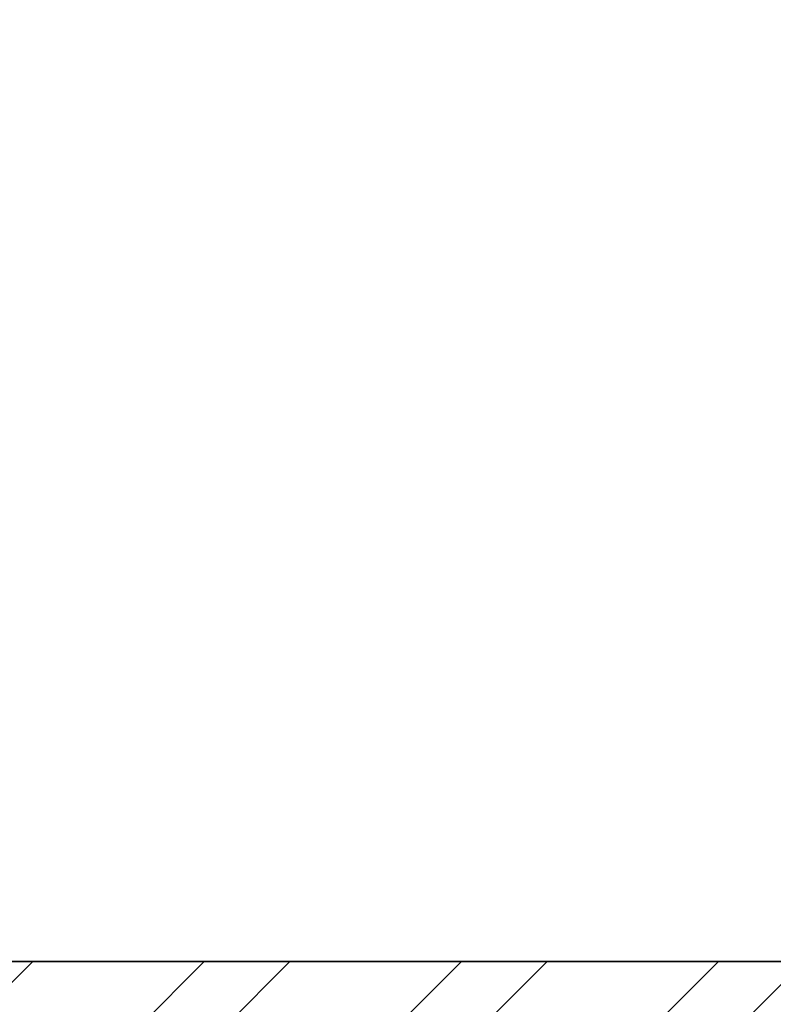
# Model space of a CAD drawing. Units: inches. Extents: x 1962 to 2771, y 1245 to 2660.
# Tile 71 of 114: x 2551 to 2590, y 1979 to 2031. Entities that reach past the tile are written whole.
import ezdxf

# ---------------------------------------------------------------- set-up
doc = ezdxf.new("R2010")
doc.units = ezdxf.units.IN
doc.layers.add('A-WALL', color=7, linetype='Continuous', lineweight=35)
doc.layers.add('A-WALL-PATT', color=252, linetype='Continuous', lineweight=13)

msp = doc.modelspace()

# ---------------------------------------------------------------- hatches: boundary and pattern name
at = {"layer": 'A-WALL-PATT'}
h = msp.add_hatch(dxfattribs=at)
h.set_pattern_fill('ANSI32', color=256)
h.paths.add_polyline_path([(2090.8074, 2467.3437), (2141.6481, 2467.3437), (2141.6481, 2469.5937), (2141.6481, 2471.8437), (2086.3074, 2471.8437), (2086.3074, 2422.5333), (2090.8074, 2422.5333)])
h.paths.add_polyline_path([(2282.7664, 2471.8437), (2204.8982, 2471.8437), (2204.8982, 2467.3437), (2234.8074, 2467.3437), (2234.8074, 2311.3437), (2228.7492, 2311.3437), (2228.7492, 2306.8437), (2234.8074, 2306.8437), (2331.9227, 2306.8437), (2331.9227, 2309.0937), (2331.9227, 2311.3437), (2239.3074, 2311.3437), (2239.3074, 2467.3437), (2282.7664, 2467.3437), (2282.7664, 2469.5937)])
h.paths.add_polyline_path([(2471.4531, 2519.8437), (2552.011, 2519.8437), (2564.3996, 2519.8437), (2564.3996, 2511.1389), (2568.8996, 2511.1389), (2568.8996, 2524.3437), (2466.9531, 2524.3437), (2466.9531, 2471.8437), (2450.0749, 2471.8437), (2446.4672, 2471.8437), (2446.4672, 2467.3437), (2450.0749, 2467.3437), (2475.9988, 2467.3437), (2475.9988, 2469.5937), (2475.9988, 2471.8437), (2471.4531, 2471.8437)])
h.paths.add_polyline_path([(2575.2231, 2469.5937), (2575.2231, 2471.8437), (2568.8996, 2471.8437), (2568.8996, 2487.1389), (2564.3996, 2487.1389), (2564.3996, 2471.8437), (2556.511, 2471.8437), (2499.2904, 2471.8437), (2499.2904, 2467.3437), (2507.8074, 2467.3437), (2507.8074, 2311.3437), (2414.863, 2311.3437), (2414.863, 2306.8437), (2512.3074, 2306.8437), (2517.0114, 2306.8437), (2517.0114, 2309.0937), (2517.0114, 2311.3437), (2512.3074, 2311.3437), (2512.3074, 2467.3437), (2575.2231, 2467.3437)])
h.paths.add_polyline_path([(2660.8074, 2471.8437), (2600.9602, 2471.8437), (2600.9602, 2467.3437), (2656.3074, 2467.3437), (2656.3074, 2432.5704), (2660.8074, 2432.5704)])
h.paths.add_polyline_path([(2660.8074, 2372.5704), (2656.3074, 2372.5704), (2656.3074, 2311.3437), (2600.276, 2311.3437), (2600.276, 2309.0937), (2600.276, 2306.8437), (2656.3074, 2306.8437), (2656.3074, 2296.2593), (2660.8074, 2296.2593)])
h.paths.add_polyline_path([(2572.3074, 2306.8437), (2577.1385, 2306.8437), (2577.1385, 2311.3437), (2551.082, 2311.3437), (2551.082, 2306.8437), (2567.8074, 2306.8437), (2567.8074, 2258.8437), (2540.0574, 2258.8437), (2540.0574, 2256.5937), (2540.0574, 2254.3437), (2567.8074, 2254.3437), (2656.3074, 2254.3437), (2656.3074, 2236.9085), (2660.8074, 2236.9085), (2660.8074, 2272.2593), (2656.3074, 2272.2593), (2656.3074, 2258.8437), (2572.3074, 2258.8437)])
h.paths.add_polyline_path([(2512.3074, 2254.3437), (2518.8716, 2254.3437), (2518.8716, 2256.5937), (2518.8716, 2258.8437), (2507.8074, 2258.8437), (2507.8074, 2177.8437), (2567.8074, 2177.8437), (2567.8074, 2172.9628), (2572.3074, 2172.9628), (2572.3074, 2177.8437), (2656.3074, 2177.8437), (2656.3074, 2166.4846), (2660.8074, 2166.4846), (2660.8074, 2200.9085), (2656.3074, 2200.9085), (2656.3074, 2182.3437), (2512.3074, 2182.3437)])
h.paths.add_polyline_path([(2656.3074, 2129.8437), (2572.3074, 2129.8437), (2572.3074, 2150.3044), (2570.0574, 2150.3044), (2567.8074, 2150.3044), (2567.8074, 2129.8437), (2507.8074, 2129.8437), (2507.8074, 2116.3027), (2510.0574, 2116.3027), (2512.3074, 2116.3027), (2512.3074, 2125.3437), (2567.8074, 2125.3437), (2572.3074, 2125.3437), (2656.3074, 2125.3437)])
h.paths.add_polyline_path([(2090.8074, 2362.5333), (2086.3074, 2362.5333), (2086.3074, 2298.6242), (2090.8074, 2298.6242), (2090.8074, 2306.8437), (2174.8074, 2306.8437), (2174.8074, 2286.4178), (2179.3074, 2286.4178), (2179.3074, 2306.8437), (2192.8641, 2306.8437), (2192.8641, 2309.0937), (2192.8641, 2311.3437), (2090.8074, 2311.3437)])
h.paths.add_polyline_path([(2209.156, 2258.8437), (2179.3074, 2258.8437), (2179.3074, 2263.2236), (2177.0574, 2263.2236), (2174.8074, 2263.2236), (2174.8074, 2258.8437), (2090.8074, 2258.8437), (2090.8074, 2274.6242), (2086.3074, 2274.6242), (2086.3074, 2238.2967), (2088.5574, 2238.2967), (2090.8074, 2238.2967), (2090.8074, 2254.3437), (2209.156, 2254.3437)])
h.paths.add_polyline_path([(2090.8074, 2177.8437), (2234.8074, 2177.8437), (2234.8074, 2173.1428), (2239.3074, 2173.1428), (2239.3074, 2258.8437), (2230.8442, 2258.8437), (2230.8442, 2256.5937), (2230.8442, 2254.3437), (2234.8074, 2254.3437), (2234.8074, 2182.3437), (2090.8074, 2182.3437), (2090.8074, 2202.2967), (2086.3074, 2202.2967), (2086.3074, 2140.0389), (2090.8074, 2140.0389)])
h.paths.add_polyline_path([(2090.8074, 2080.0389), (2086.3074, 2080.0389), (2086.3074, 2033.8437), (2090.8074, 2033.8437)], flags=17)
h.paths.add_polyline_path([(2244.9405, 2033.8437), (2239.3074, 2033.8437), (2239.3074, 2142.0665), (2237.2592, 2142.0665), (2234.8074, 2142.0665), (2234.8074, 2033.8437), (2090.8074, 2033.8437), (2076.5204, 2033.8437), (2072.0204, 2033.8437), (2072.0204, 2000.4493), (2076.5204, 2000.4493), (2076.5204, 2029.3437), (2090.8074, 2029.3437), (2244.9405, 2029.3437), (2244.9405, 2031.5937)])
h.paths.add_polyline_path([(2234.8074, 1933.3437), (2076.5204, 1933.3437), (2076.5204, 1952.4493), (2074.2704, 1952.4493), (2072.0204, 1952.4493), (2072.0204, 1933.3437), (2072.0204, 1928.8437), (2234.8074, 1928.8437)])
h.paths.add_polyline_path([(2090.8074, 1928.8437), (2086.3074, 1928.8437), (2086.3074, 1906.5013), (2090.8074, 1906.5013)])
h.paths.add_polyline_path([(2090.8074, 1846.5013), (2086.3074, 1846.5013), (2086.3074, 1769.9917), (2088.5574, 1769.9917), (2090.8074, 1769.9917), (2090.8074, 1780.3437), (2234.8074, 1780.3437), (2234.8074, 1708.3437), (2230.3764, 1708.3437), (2230.3764, 1703.8437), (2239.3074, 1703.8437), (2239.3074, 1792.6669), (2237.0574, 1792.6669), (2234.8074, 1792.6669), (2234.8074, 1784.8437), (2090.8074, 1784.8437)])
h.paths.add_polyline_path([(2239.3074, 1928.8437), (2244.9405, 1928.8437), (2244.9405, 1931.0937), (2244.9405, 1933.3437), (2234.8074, 1933.3437), (2234.8074, 1928.8437), (2234.8074, 1825.5949), (2239.3074, 1825.5949)])
h.paths.add_polyline_path([(2148.0425, 1649.0937), (2148.0425, 1651.3437), (2090.8074, 1651.3437), (2090.8074, 1646.8437), (2148.0425, 1646.8437)], flags=0)
h.paths.add_polyline_path([(2207.5601, 1708.3437), (2090.8074, 1708.3437), (2090.8074, 1703.8437), (2174.8074, 1703.8437), (2174.8074, 1651.3437), (2170.4457, 1651.3437), (2170.4457, 1646.8437), (2195.9924, 1646.8437), (2195.9924, 1649.0937), (2195.9924, 1651.3437), (2179.3074, 1651.3437), (2179.3074, 1703.8437), (2207.5601, 1703.8437), (2207.5601, 1706.0937)])
h.paths.add_polyline_path([(2090.8074, 1733.9917), (2086.3074, 1733.9917), (2086.3074, 1696.1032), (2088.5574, 1696.1032), (2090.8074, 1696.1032)])
h.paths.add_polyline_path([(2090.8074, 1672.1032), (2086.3074, 1672.1032), (2086.3074, 1600.3335), (2090.8074, 1600.3335)])
h.paths.add_polyline_path([(2090.8074, 1540.3335), (2086.3074, 1540.3335), (2086.3074, 1486.3437), (2139.6766, 1486.3437), (2139.6766, 1490.8437), (2090.8074, 1490.8437)])
h.paths.add_polyline_path([(2302.3876, 1490.8437), (2239.3074, 1490.8437), (2239.3074, 1646.8437), (2335.9994, 1646.8437), (2335.9994, 1651.3437), (2229.884, 1651.3437), (2229.884, 1646.8437), (2234.8074, 1646.8437), (2234.8074, 1490.8437), (2202.7103, 1490.8437), (2202.7103, 1488.5937), (2202.7103, 1486.3437), (2275.0699, 1486.3437), (2275.0699, 1475.772), (2279.5699, 1475.772), (2279.5699, 1486.3437), (2302.3876, 1486.3437)])
h.paths.add_polyline_path([(2279.5699, 1451.772), (2275.0699, 1451.772), (2275.0699, 1438.3437), (2174.8074, 1438.3437), (2174.8074, 1486.3437), (2179.7922, 1486.3437), (2179.7922, 1490.8437), (2163.3585, 1490.8437), (2163.3585, 1488.5937), (2163.3585, 1486.3437), (2170.3074, 1486.3437), (2170.3074, 1433.8437), (2279.5699, 1433.8437)])
h.paths.add_polyline_path([(2427.2363, 1490.8437), (2375.8074, 1490.8437), (2375.8074, 1646.8437), (2381.6401, 1646.8437), (2381.6401, 1651.3437), (2365.887, 1651.3437), (2365.887, 1649.0937), (2365.887, 1646.8437), (2371.3074, 1646.8437), (2371.3074, 1490.8437), (2327.5627, 1490.8437), (2327.5627, 1488.5937), (2327.5627, 1486.3437), (2371.3074, 1486.3437), (2371.3074, 1433.8437), (2375.8074, 1433.8437), (2375.8074, 1486.3437), (2427.2363, 1486.3437)])
h.paths.add_polyline_path([(2512.3074, 1646.8437), (2519.4351, 1646.8437), (2519.4351, 1649.0937), (2519.4351, 1651.3437), (2507.8074, 1651.3437), (2416.0063, 1651.3437), (2416.0063, 1649.0937), (2416.0063, 1646.8437), (2507.8074, 1646.8437), (2507.8074, 1490.8437), (2497.0532, 1490.8437), (2497.0532, 1488.5937), (2497.0532, 1486.3437), (2574.9344, 1486.3437), (2574.9344, 1476.0181), (2579.4344, 1476.0181), (2579.4344, 1486.3437), (2584.4872, 1486.3437), (2584.3074, 1490.8437), (2512.3074, 1490.8437)])
h.paths.add_polyline_path([(2470.5091, 1486.3437), (2473.9767, 1486.3437), (2473.9767, 1490.8437), (2449.6605, 1490.8437), (2449.6605, 1488.5937), (2449.6605, 1486.3437), (2466.0091, 1486.3437), (2466.0091, 1433.8437), (2470.5091, 1433.8437), (2579.4344, 1433.8437), (2579.4344, 1452.0181), (2574.9344, 1452.0181), (2574.9344, 1438.3437), (2554.5091, 1438.3437), (2470.5091, 1438.3437)])
h.paths.add_polyline_path([(2656.3074, 1490.8437), (2611.86, 1490.8437), (2611.86, 1486.3437), (2656.3074, 1486.3437)])
h.paths.add_polyline_path([(2660.8074, 1532.7007), (2658.5574, 1532.7007), (2656.3074, 1532.7007), (2656.3074, 1486.3437), (2660.8074, 1486.3437)])
h.paths.add_polyline_path([(2660.8074, 1664.9663), (2656.3074, 1664.9663), (2656.3074, 1651.3437), (2602.2313, 1651.3437), (2602.2313, 1646.8437), (2656.3074, 1646.8437), (2656.3074, 1592.7007), (2660.8074, 1592.7007)])
h.paths.add_polyline_path([(2660.8074, 1724.5221), (2656.3074, 1724.5221), (2656.3074, 1703.8437), (2542.4725, 1703.8437), (2542.4725, 1699.3437), (2567.8074, 1699.3437), (2567.8074, 1651.3437), (2552.7766, 1651.3437), (2552.7766, 1649.0937), (2552.7766, 1646.8437), (2577.2878, 1646.8437), (2577.2878, 1649.0937), (2577.2878, 1651.3437), (2572.3074, 1651.3437), (2572.3074, 1699.3437), (2656.3074, 1699.3437), (2656.3074, 1688.9663), (2660.8074, 1688.9663)])
h.paths.add_polyline_path([(2660.8074, 1880.6524), (2656.3074, 1880.6524), (2656.3074, 1832.8437), (2512.3074, 1832.8437), (2512.3074, 1837.8959), (2507.8074, 1837.8959), (2507.8074, 1828.3437), (2567.8074, 1828.3437), (2567.8074, 1804.3437), (2572.3074, 1804.3437), (2572.3074, 1828.3437), (2656.3074, 1828.3437), (2656.3074, 1818.6778), (2660.8074, 1818.6778)])
h.paths.add_polyline_path([(2660.8074, 1794.6778), (2656.3074, 1794.6778), (2656.3074, 1780.3437), (2572.3074, 1780.3437), (2572.3074, 1783.0303), (2570.0574, 1783.0303), (2567.8074, 1783.0303), (2567.8074, 1780.3437), (2507.8074, 1780.3437), (2507.8074, 1699.3437), (2517.8858, 1699.3437), (2517.8858, 1701.5937), (2517.8858, 1703.8437), (2512.3074, 1703.8437), (2512.3074, 1775.8437), (2656.3074, 1775.8437), (2656.3074, 1760.5221), (2660.8074, 1760.5221)])
h.paths.add_polyline_path([(2660.8074, 1981.3437), (2660.8074, 2020.2808), (2658.5574, 2020.2808), (2656.3074, 2020.2808), (2656.3074, 1981.3437), (2512.3074, 1981.3437), (2512.3074, 2086.6996), (2507.8074, 2086.6996), (2507.8074, 1981.3437), (2375.8074, 1981.3437), (2375.8074, 1986.8505), (2373.5574, 1986.8505), (2371.3074, 1986.8505), (2371.3074, 1973.2607), (2375.8074, 1973.2607), (2375.8074, 1976.8437), (2507.8074, 1976.8437), (2507.8074, 1865.4281), (2510.0574, 1865.4281), (2512.3074, 1865.4281), (2512.3074, 1976.8437), (2660.8074, 1976.8437)])
h.paths.add_polyline_path([(2375.8074, 1940.297), (2373.5574, 1940.297), (2371.3074, 1940.297), (2371.3074, 1933.3437), (2278.4434, 1933.3437), (2278.4434, 1928.8437), (2371.3074, 1928.8437), (2371.3074, 1651.3437), (2375.8074, 1651.3437)])
h.paths.add_polyline_path([(2660.8074, 1976.8437), (2656.3074, 1976.8437), (2656.3074, 1940.6524), (2660.8074, 1940.6524)], flags=17)
h.paths.add_polyline_path([(2660.8074, 2142.4846), (2656.3074, 2142.4846), (2656.3074, 2080.2808), (2660.8074, 2080.2808)])
h.paths.add_polyline_path([(2381.4189, 2311.3437), (2375.8074, 2311.3437), (2375.8074, 2467.3437), (2424.7242, 2467.3437), (2424.7242, 2469.5937), (2424.7242, 2471.8437), (2375.8074, 2471.8437), (2375.8074, 2524.3437), (2371.3074, 2524.3437), (2371.3074, 2471.8437), (2307.2097, 2471.8437), (2307.2097, 2467.3437), (2371.3074, 2467.3437), (2371.3074, 2311.3437), (2366.8901, 2311.3437), (2366.8901, 2306.8437), (2371.3074, 2306.8437), (2371.3074, 2033.8437), (2279.6589, 2033.8437), (2279.6589, 2029.3437), (2371.3074, 2029.3437), (2371.3074, 2014.2598), (2375.8074, 2014.2598), (2375.8074, 2306.8437), (2381.4189, 2306.8437)])
h.paths.add_polyline_path([(2263.3074, 2524.3437), (2170.3074, 2524.3437), (2170.3074, 2519.8437), (2170.3074, 2471.8437), (2165.0312, 2471.8437), (2165.0312, 2467.3437), (2179.6721, 2467.3437), (2179.6721, 2469.5161), (2179.6721, 2471.8437), (2174.8074, 2471.8437), (2174.8074, 2519.8437), (2258.8074, 2519.8437), (2258.8074, 2511.6436), (2263.3074, 2511.6436)])
h.paths.add_polyline_path([(2245.0232, 1361.4123), (2492.9468, 1361.4123), (2492.9468, 1398.505), (2245.0232, 1398.505)], flags=9)
h.paths.add_polyline_path([(2388.1434, 2086.6936), (2425.0704, 2086.6936), (2425.0704, 2105.3509), (2388.1434, 2105.3509)], flags=9)
h.paths.add_polyline_path([(2404.922, 2242.6744), (2445.7337, 2242.6744), (2445.7337, 2261.3318), (2404.922, 2261.3318)], flags=9)
h.paths.add_polyline_path([(2269.4107, 2156.7935), (2306.3378, 2156.7935), (2306.3378, 2175.4508), (2269.4107, 2175.4508)], flags=9)
h.paths.add_polyline_path([(2269.3277, 2233.4343), (2306.2547, 2233.4343), (2306.2547, 2252.0917), (2269.3277, 2252.0917)], flags=9)
h.paths.add_polyline_path([(2431.6052, 2320.6922), (2470.4456, 2320.6922), (2470.4456, 2339.3495), (2431.6052, 2339.3495)], flags=25)
h.paths.add_polyline_path([(2249.6902, 2315.7608), (2288.5306, 2315.7608), (2288.5306, 2334.4182), (2249.6902, 2334.4182)], flags=25)
h.paths.add_polyline_path([(2096.9301, 2314.3181), (2135.7704, 2314.3181), (2135.7704, 2332.9755), (2096.9301, 2332.9755)], flags=25)
h.paths.add_polyline_path([(2134.3475, 2285.7089), (2161.4655, 2285.7089), (2161.4655, 2304.3662), (2134.3475, 2304.3662)], flags=9)
h.paths.add_polyline_path([(2126.5155, 2209.4076), (2159.9227, 2209.4076), (2159.9227, 2228.065), (2126.5155, 2228.065)], flags=25)
h.paths.add_polyline_path([(2110.5753, 2141.5299), (2149.4157, 2141.5299), (2149.4157, 2160.1872), (2110.5753, 2160.1872)], flags=25)
h.paths.add_polyline_path([(2249.8618, 1968.3317), (2286.3966, 1968.3317), (2286.3966, 1986.989), (2249.8618, 1986.989)], flags=9)
h.paths.add_polyline_path([(2395.9507, 1777.0051), (2436.7624, 1777.0051), (2436.7624, 1795.6625), (2395.9507, 1795.6625)], flags=9)
h.paths.add_polyline_path([(2398.5259, 1888.5651), (2435.0062, 1888.5651), (2435.0062, 1907.2224), (2398.5259, 1907.2224)], flags=25)
h.paths.add_polyline_path([(2259.3506, 1728.3559), (2296.2776, 1728.3559), (2296.2776, 1747.0132), (2259.3506, 1747.0132)], flags=9)
h.paths.add_polyline_path([(2271.3698, 1845.268), (2308.2968, 1845.268), (2308.2968, 1863.9253), (2271.3698, 1863.9253)], flags=9)
h.paths.add_polyline_path([(2120.9355, 1786.3027), (2159.7759, 1786.3027), (2159.7759, 1804.9601), (2120.9355, 1804.9601)], flags=25)
h.paths.add_polyline_path([(2121.3164, 1732.1043), (2154.7236, 1732.1043), (2154.7236, 1750.7616), (2121.3164, 1750.7616)], flags=25)
h.paths.add_polyline_path([(2118.3706, 1678.8997), (2147.5282, 1678.8997), (2147.5282, 1697.557), (2118.3706, 1697.557)], flags=25)
h.paths.add_polyline_path([(2385.9227, 1493.557), (2424.763, 1493.557), (2424.763, 1512.2143), (2385.9227, 1512.2143)], flags=25)
h.paths.add_polyline_path([(2248.7058, 1500.0256), (2287.5462, 1500.0256), (2287.5462, 1518.6829), (2248.7058, 1518.6829)], flags=25)
h.paths.add_polyline_path([(2104.1669, 1617.3771), (2143.0073, 1617.3771), (2143.0073, 1636.0344), (2104.1669, 1636.0344)], flags=9)
h.paths.add_polyline_path([(2096.0714, 1447.8824), (2137.3845, 1447.8824), (2137.3845, 1458.1859), (2096.0714, 1458.1859)], flags=9)
h.paths.add_polyline_path([(2180.6114, 1440.325), (2209.7689, 1440.325), (2209.7689, 1458.9823), (2180.6114, 1458.9823)], flags=25)
h.paths.add_polyline_path([(2316.1698, 1447.9637), (2357.4829, 1447.9637), (2357.4829, 1458.2673), (2316.1698, 1458.2673)], flags=9)
h.paths.add_polyline_path([(2397.6187, 1447.9637), (2438.9318, 1447.9637), (2438.9318, 1458.2673), (2397.6187, 1458.2673)], flags=9)
h.paths.add_polyline_path([(2473.0778, 1439.5953), (2502.2354, 1439.5953), (2502.2354, 1458.2527), (2473.0778, 1458.2527)], flags=25)
h.paths.add_polyline_path([(2589.7027, 1447.8819), (2631.0158, 1447.8819), (2631.0158, 1458.1855), (2589.7027, 1458.1855)], flags=9)
h.paths.add_polyline_path([(2522.4009, 1497.5285), (2561.2413, 1497.5285), (2561.2413, 1516.1859), (2522.4009, 1516.1859)], flags=25)
h.paths.add_polyline_path([(2579.6565, 1671.3482), (2608.8141, 1671.3482), (2608.8141, 1690.0056), (2579.6565, 1690.0056)], flags=25)
h.paths.add_polyline_path([(2544.7038, 1725.5064), (2578.1111, 1725.5064), (2578.1111, 1744.1637), (2544.7038, 1744.1637)], flags=25)
h.paths.add_polyline_path([(2578.1191, 1807.472), (2607.2766, 1807.472), (2607.2766, 1826.1293), (2578.1191, 1826.1293)], flags=25)
h.paths.add_polyline_path([(2595.0614, 1835.1839), (2633.9018, 1835.1839), (2633.9018, 1853.8413), (2595.0614, 1853.8413)], flags=25)
h.paths.add_polyline_path([(2567.0097, 2097.7035), (2605.8501, 2097.7035), (2605.8501, 2116.3609), (2567.0097, 2116.3609)], flags=9)
h.paths.add_polyline_path([(2586.644, 2134.6454), (2615.8015, 2134.6454), (2615.8015, 2153.3027), (2586.644, 2153.3027)], flags=9)
h.paths.add_polyline_path([(2544.6185, 2212.6783), (2578.0258, 2212.6783), (2578.0258, 2231.3356), (2544.6185, 2231.3356)], flags=25)
h.paths.add_polyline_path([(2577.0273, 2256.9023), (2606.1849, 2256.9023), (2606.1849, 2275.5597), (2577.0273, 2275.5597)], flags=24)
h.paths.add_polyline_path([(2605.2683, 2315.2821), (2644.1087, 2315.2821), (2644.1087, 2333.9395), (2605.2683, 2333.9395)], flags=25)
h.paths.add_polyline_path([(2583.1244, 2496.1815), (2624.4375, 2496.1815), (2624.4375, 2506.4851), (2583.1244, 2506.4851)], flags=9)
h.paths.add_polyline_path([(2474.761, 2497.0823), (2503.9185, 2497.0823), (2503.9185, 2515.7397), (2474.761, 2515.7397)], flags=25)
h.paths.add_polyline_path([(2387.5787, 2494.2563), (2428.902, 2494.2563), (2428.902, 2504.5598), (2387.5787, 2504.5598)], flags=9)
h.paths.add_polyline_path([(2300.1657, 2500.1564), (2341.4788, 2500.1564), (2341.4788, 2510.46), (2300.1657, 2510.46)], flags=25)
h.paths.add_polyline_path([(2176.8589, 2497.5843), (2206.0165, 2497.5843), (2206.0165, 2516.2416), (2176.8589, 2516.2416)], flags=25)
h.paths.add_polyline_path([(2097.4668, 2494.9762), (2138.7799, 2494.9762), (2138.7799, 2505.2798), (2097.4668, 2505.2798)], flags=9)

# ---------------------------------------------------------------- linework, layer by layer
at = {"layer": 'A-WALL'}
msp.add_line((2512.3074, 1981.3437), (2656.3074, 1981.3437), dxfattribs=at)

doc.saveas('drawing.dxf')
